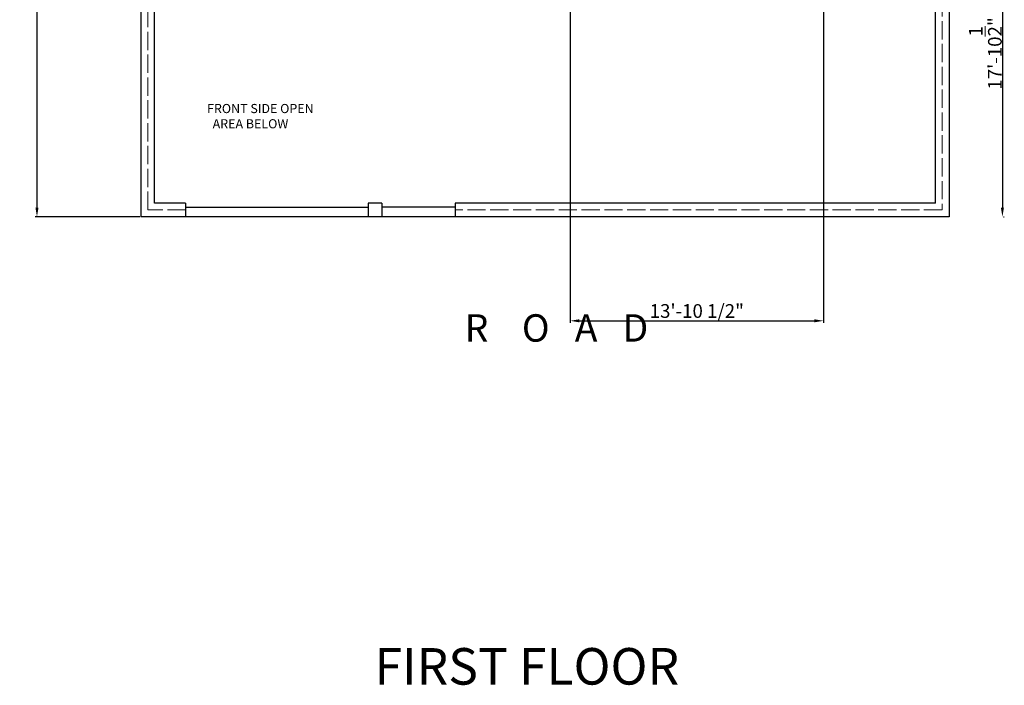
# Model space of a CAD drawing. Units: millimetres. Extents: x 595116 to 630915, y 909473 to 920225.
# Tile 127 of 134: x 630214 to 630861, y 918839 to 919276. Entities that reach past the tile are written whole.
import ezdxf

# ---------------------------------------------------------------- set-up
doc = ezdxf.new("R2010")
doc.units = ezdxf.units.MM
doc.linetypes.add('ACAD_ISO02W100', pattern=[15, 12, -3])
for name, color, linetype, lineweight in [('A-ANNO-TITL', 7, 'Continuous', 35), ('A-AREA-IDEN', 7, 'Continuous', 20), ('C-PROP', 7, 'Continuous', 25), ('C-PROP-REF', 240, 'ACAD_ISO02W100', 13), ('Dimension', 3, 'Continuous', 18), ('Text', 7, 'Continuous', 18)]:
    doc.layers.add(name, color=color, linetype=linetype, lineweight=lineweight)
doc.styles.get("Standard").update_dxf_attribs({"font": 'arial.ttf'})
doc.dimstyles.new('ISO-25', dxfattribs={"dimtxt": 9, "dimasz": 6, "dimexe": 1.25, "dimexo": 0.625, "dimtad": 1, "dimlunit": 4, "dimtxsty": 'Standard', "dimcen": 2.5, "dimadec": 0, "dimazin": 0, "dimtfac": 1, "dimtmove": 0, "dimatfit": 3, "dimfxl": 1, "dimarcsym": 0})

# ---------------------------------------------------------------- blocks, each defined once
blk = doc.blocks.new('*D132')
at = {"layer": 'Defpoints', "color": 0, "transparency": 16777216}
for p in [(630859.62, 919360.93), (630859.62, 919146.43), (630859.62, 919146.43)]:
    blk.add_point(p, dxfattribs=at)
at = {"layer": 'Dimension', "color": 0, "lineweight": -2, "transparency": 16777216}
for p, q in [((630860.25, 919360.93), (630860.87, 919360.93)), ((630859.62, 919354.93), (630859.62, 919152.43)), ((630860.25, 919146.43), (630860.87, 919146.43))]:
    blk.add_line(p, q, dxfattribs=at)
at = {"layer": 'Dimension', "color": 0, "transparency": 16777216}
for points in [[(630858.62, 919354.93), (630860.62, 919354.93), (630859.62, 919360.93)], [(630858.62, 919152.43), (630860.62, 919152.43), (630859.62, 919146.43)]]:
    blk.add_solid(points, dxfattribs=at)
at = {"layer": 'Dimension', "color": 0, "transparency": 16777216, "insert": (630848.38, 919253.68), "char_height": 9, "attachment_point": 5, "rotation": 90}
blk.add_mtext('17\'-10{\\H1x;\\S1/2;}"', dxfattribs=at)
blk = doc.blocks.new('*D214')
at = {"layer": 'Defpoints', "color": 0, "transparency": 16777216}
for p in [(630293.6, 920089.43), (630225.3, 919146.43), (630293.6, 919146.43)]:
    blk.add_point(p, dxfattribs=at)
at = {"layer": 'Dimension', "color": 0, "lineweight": -2, "transparency": 16777216}
for p, q in [((630292.97, 920089.43), (630224.05, 920089.43)), ((630225.3, 920083.43), (630225.3, 919152.43)), ((630292.97, 919146.43), (630224.05, 919146.43))]:
    blk.add_line(p, q, dxfattribs=at)
at = {"layer": 'Dimension', "color": 0, "transparency": 16777216}
for points in [[(630224.3, 920083.43), (630226.3, 920083.43), (630225.3, 920089.43)], [(630224.3, 919152.43), (630226.3, 919152.43), (630225.3, 919146.43)]]:
    blk.add_solid(points, dxfattribs=at)
at = {"layer": 'Dimension', "color": 0, "transparency": 16777216, "insert": (630220.08, 919617.93), "char_height": 9, "attachment_point": 5, "rotation": 90}
blk.add_mtext('78\'-7"', dxfattribs=at)
blk = doc.blocks.new('*D218')
at = {"layer": 'Defpoints', "color": 0, "transparency": 16777216}
for p in [(630575.6, 919333.93), (630742.1, 919333.93), (630742.1, 919078.13)]:
    blk.add_point(p, dxfattribs=at)
at = {"layer": 'Dimension', "color": 0, "lineweight": -2, "transparency": 16777216}
for p, q in [((630575.6, 919333.3), (630575.6, 919076.88)), ((630742.1, 919333.3), (630742.1, 919076.88)), ((630581.6, 919078.13), (630736.1, 919078.13))]:
    blk.add_line(p, q, dxfattribs=at)
at = {"layer": 'Dimension', "color": 0, "transparency": 16777216}
for points in [[(630581.6, 919079.13), (630581.6, 919077.13), (630575.6, 919078.13)], [(630736.1, 919079.13), (630736.1, 919077.13), (630742.1, 919078.13)]]:
    blk.add_solid(points, dxfattribs=at)
at = {"layer": 'Dimension', "color": 0, "transparency": 16777216, "insert": (630658.85, 919083.41), "char_height": 9, "attachment_point": 5}
blk.add_mtext('13\'-10 1/2"', dxfattribs=at)

msp = doc.modelspace()

# ---------------------------------------------------------------- linework, layer by layer
at = {"layer": 'C-PROP'}
for p, q in [((630293.596, 919516.015), (630293.596, 919146.428)), ((630302.596, 919155.428), (630302.596, 919429.828)), ((630815.596, 919155.428), (630815.596, 919333.928)), ((630824.596, 919333.928), (630824.596, 919146.428)), ((630322.984, 919155.428), (630302.596, 919155.428)), ((630322.984, 919155.428), (630322.984, 919146.428)), ((630322.984, 919152.681), (630442.984, 919152.681)), ((630442.984, 919155.428), (630442.984, 919146.428)), ((630451.984, 919155.428), (630442.984, 919155.428)), ((630451.984, 919155.428), (630451.984, 919146.428)), ((630451.984, 919152.943), (630499.984, 919152.943)), ((630815.596, 919155.428), (630499.984, 919155.428)), ((630499.984, 919155.428), (630499.984, 919146.428))]:
    msp.add_line(p, q, dxfattribs=at)
msp.add_lwpolyline([(630824.596, 919146.428), (630293.596, 919146.428)], dxfattribs=at)
at = {"layer": 'C-PROP-REF'}
for p, q in [((630298.096, 919150.928), (630298.096, 920084.928)), ((630820.096, 920084.928), (630820.096, 919150.928)), ((630322.984, 919150.928), (630298.096, 919150.928)), ((630820.096, 919150.928), (630499.984, 919150.928))]:
    msp.add_line(p, q, dxfattribs=at)

# ---------------------------------------------------------------- texts
at = {"layer": 'A-ANNO-TITL', "insert": (630395.732, 918863.187), "char_height": 24, "attachment_point": 1, "rotation": 0.018333}
msp.add_mtext_dynamic_manual_height_columns('{       FIRST FLOOR}', width=350.55928, gutter_width=12.5, heights=[0], dxfattribs=at)
at = {"layer": 'A-AREA-IDEN', "insert": (630337.064, 919220.513), "char_height": 6, "attachment_point": 1}
msp.add_mtext_dynamic_manual_height_columns('{FRONT SIDE OPEN\\P  AREA BELOW}', width=125.26422, gutter_width=12.5, heights=[0], dxfattribs=at)
at = {"layer": 'Text', "insert": (630506.303, 919082.405), "char_height": 18, "attachment_point": 1, "rotation": 0.018333}
msp.add_mtext_dynamic_manual_height_columns('{R    O   A   D}', width=269.48254, gutter_width=12.5, heights=[0], dxfattribs=at)

# ---------------------------------------------------------------- dimensions: what is measured, and where the dimension line sits
at = {"layer": 'Dimension'}
for base, p1, p2, override, picture, middle in [((630225.296, 919146.428), (630293.596, 920089.428), (630293.596, 919146.428), {"dimdec": 1, "dimlfac": 1, "dimrnd": 0, "dimzin": 1, "dimdsep": 46, "dimlunit": 4, "dimfrac": 2}, '*D214', (630220.076, 919617.928)), ((630859.621, 919146.428), (630859.621, 919360.928), (630859.621, 919146.428), {"dimclrd": 0, "dimclre": 0, "dimclrt": 0}, '*D132', (630848.383, 919253.678))]:
    dim = msp.add_linear_dim(base=base, p1=p1, p2=p2, angle=90, dimstyle='ISO-25', override=override, dxfattribs=at)
    dim.commit()
    dim.dimension.update_dxf_attribs({"geometry": picture, "text_midpoint": middle})
dim = msp.add_linear_dim(base=(630742.096, 919078.128), p1=(630575.596, 919333.928), p2=(630742.096, 919333.928), dimstyle='ISO-25', override={"dimdec": 1, "dimlfac": 1, "dimrnd": 0, "dimzin": 1, "dimdsep": 46, "dimlunit": 4, "dimfrac": 2}, dxfattribs=at)
dim.commit()
dim.dimension.update_dxf_attribs({"geometry": '*D218', "text_midpoint": (630658.846, 919083.409)})

doc.saveas('drawing.dxf')
